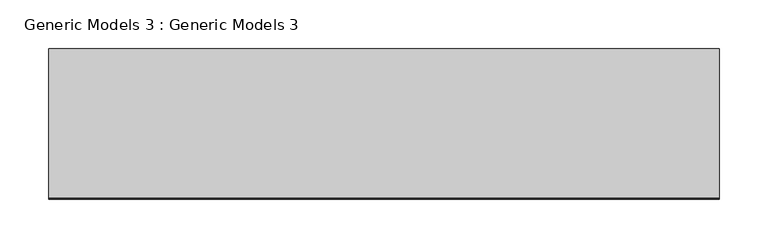
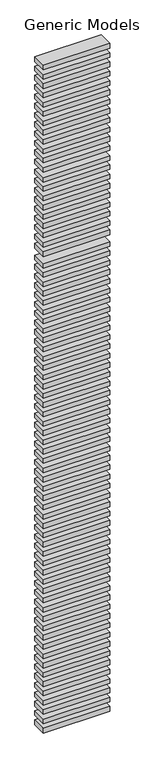
"""IFC4 building model written with IfcOpenShell, lengths in millimetres: proxy geometry, Generic Models 3 : Generic Models 3."""

from ifc_helpers import new_model, si_unit, frame, origin, place, context, project, spatial, polyline, outline, extrude, source, transform, mapped, element, save


def generic_models_3_generic_models_3_1afd715e(model_context):
    return source(origin(), model_context, "Body", "SweptSolid", [
        extrude(outline(polyline([(8219.67371, -13654.3073314), (7533.87371, -13654.3073314), (7533.87371, -13501.9073314), (8219.67371, -13501.9073314), (8219.67371, -13654.3073314)])), frame((0.0, 0.0, 7618.979075), z_axis=(0.0, 0.0, 1.0), x_axis=(1.0, 0.0, 0.0)), (0.0, 0.0, 1.0), 50.8),
        extrude(outline(polyline([(8219.67371, -13654.3073314), (7533.87371, -13654.3073314), (7533.87371, -13501.9073314), (8219.67371, -13501.9073314), (8219.67371, -13654.3073314)])), frame((0.0, 0.0, 7517.379075), z_axis=(0.0, 0.0, 1.0), x_axis=(1.0, 0.0, 0.0)), (0.0, 0.0, 1.0), 50.8),
        extrude(outline(polyline([(8219.67371, -13654.3073314), (7533.87371, -13654.3073314), (7533.87371, -13501.9073314), (8219.67371, -13501.9073314), (8219.67371, -13654.3073314)])), frame((0.0, 0.0, 7415.779075), z_axis=(0.0, 0.0, 1.0), x_axis=(1.0, 0.0, 0.0)), (0.0, 0.0, 1.0), 50.8),
        extrude(outline(polyline([(8219.67371, -13654.3073314), (7533.87371, -13654.3073314), (7533.87371, -13501.9073314), (8219.67371, -13501.9073314), (8219.67371, -13654.3073314)])), frame((0.0, 0.0, 7314.179075), z_axis=(0.0, 0.0, 1.0), x_axis=(1.0, 0.0, 0.0)), (0.0, 0.0, 1.0), 50.8),
        extrude(outline(polyline([(8219.67371, -13654.3073314), (7533.87371, -13654.3073314), (7533.87371, -13501.9073314), (8219.67371, -13501.9073314), (8219.67371, -13654.3073314)])), frame((0.0, 0.0, 7212.579075), z_axis=(0.0, 0.0, 1.0), x_axis=(1.0, 0.0, 0.0)), (0.0, 0.0, 1.0), 50.8),
        extrude(outline(polyline([(8219.67371, -13654.3073314), (7533.87371, -13654.3073314), (7533.87371, -13501.9073314), (8219.67371, -13501.9073314), (8219.67371, -13654.3073314)])), frame((0.0, 0.0, 7110.979075), z_axis=(0.0, 0.0, 1.0), x_axis=(1.0, 0.0, 0.0)), (0.0, 0.0, 1.0), 50.8),
        extrude(outline(polyline([(8219.67371, -13654.3073314), (7533.87371, -13654.3073314), (7533.87371, -13501.9073314), (8219.67371, -13501.9073314), (8219.67371, -13654.3073314)])), frame((0.0, 0.0, 7009.379075), z_axis=(0.0, 0.0, 1.0), x_axis=(1.0, 0.0, 0.0)), (0.0, 0.0, 1.0), 50.8),
        extrude(outline(polyline([(8219.67371, -13654.3073314), (7533.87371, -13654.3073314), (7533.87371, -13501.9073314), (8219.67371, -13501.9073314), (8219.67371, -13654.3073314)])), frame((0.0, 0.0, 6907.779075), z_axis=(0.0, 0.0, 1.0), x_axis=(1.0, 0.0, 0.0)), (0.0, 0.0, 1.0), 50.8),
        extrude(outline(polyline([(8219.67371, -13654.3073314), (7533.87371, -13654.3073314), (7533.87371, -13501.9073314), (8219.67371, -13501.9073314), (8219.67371, -13654.3073314)])), frame((0.0, 0.0, 6806.179075), z_axis=(0.0, 0.0, 1.0), x_axis=(1.0, 0.0, 0.0)), (0.0, 0.0, 1.0), 50.8),
        extrude(outline(polyline([(8219.67371, -13654.3073314), (7533.87371, -13654.3073314), (7533.87371, -13501.9073314), (8219.67371, -13501.9073314), (8219.67371, -13654.3073314)])), frame((0.0, 0.0, 6704.579075), z_axis=(0.0, 0.0, 1.0), x_axis=(1.0, 0.0, 0.0)), (0.0, 0.0, 1.0), 50.8),
        extrude(outline(polyline([(8219.67371, -13654.3073314), (7533.87371, -13654.3073314), (7533.87371, -13501.9073314), (8219.67371, -13501.9073314), (8219.67371, -13654.3073314)])), frame((0.0, 0.0, 6602.979075), z_axis=(0.0, 0.0, 1.0), x_axis=(1.0, 0.0, 0.0)), (0.0, 0.0, 1.0), 50.8),
        extrude(outline(polyline([(8219.67371, -13654.3073314), (7533.87371, -13654.3073314), (7533.87371, -13501.9073314), (8219.67371, -13501.9073314), (8219.67371, -13654.3073314)])), frame((0.0, 0.0, 6501.379075), z_axis=(0.0, 0.0, 1.0), x_axis=(1.0, 0.0, 0.0)), (0.0, 0.0, 1.0), 50.8),
        extrude(outline(polyline([(8219.67371, -13654.3073314), (7533.87371, -13654.3073314), (7533.87371, -13501.9073314), (8219.67371, -13501.9073314), (8219.67371, -13654.3073314)])), frame((0.0, 0.0, 6393.429075), z_axis=(0.0, 0.0, 1.0), x_axis=(1.0, 0.0, 0.0)), (0.0, 0.0, 1.0), 50.8),
        extrude(outline(polyline([(8219.67371, -13654.3073314), (7533.87371, -13654.3073314), (7533.87371, -13501.9073314), (8219.67371, -13501.9073314), (8219.67371, -13654.3073314)])), frame((0.0, 0.0, 6291.829075), z_axis=(0.0, 0.0, 1.0), x_axis=(1.0, 0.0, 0.0)), (0.0, 0.0, 1.0), 50.8),
        extrude(outline(polyline([(8219.67371, -13654.3073314), (7533.87371, -13654.3073314), (7533.87371, -13501.9073314), (8219.67371, -13501.9073314), (8219.67371, -13654.3073314)])), frame((0.0, 0.0, 6190.229075), z_axis=(0.0, 0.0, 1.0), x_axis=(1.0, 0.0, 0.0)), (0.0, 0.0, 1.0), 50.8),
        extrude(outline(polyline([(8219.67371, -13654.3073314), (7533.87371, -13654.3073314), (7533.87371, -13501.9073314), (8219.67371, -13501.9073314), (8219.67371, -13654.3073314)])), frame((0.0, 0.0, 6088.629075), z_axis=(0.0, 0.0, 1.0), x_axis=(1.0, 0.0, 0.0)), (0.0, 0.0, 1.0), 50.8),
        extrude(outline(polyline([(8219.67371, -13654.3073314), (7533.87371, -13654.3073314), (7533.87371, -13501.9073314), (8219.67371, -13501.9073314), (8219.67371, -13654.3073314)])), frame((0.0, 0.0, 5987.029075), z_axis=(0.0, 0.0, 1.0), x_axis=(1.0, 0.0, 0.0)), (0.0, 0.0, 1.0), 50.8),
        extrude(outline(polyline([(8219.67371, -13654.3073314), (7533.87371, -13654.3073314), (7533.87371, -13501.9073314), (8219.67371, -13501.9073314), (8219.67371, -13654.3073314)])), frame((0.0, 0.0, 5885.429075), z_axis=(0.0, 0.0, 1.0), x_axis=(1.0, 0.0, 0.0)), (0.0, 0.0, 1.0), 50.8),
        extrude(outline(polyline([(8219.67371, -13654.3073314), (7533.87371, -13654.3073314), (7533.87371, -13501.9073314), (8219.67371, -13501.9073314), (8219.67371, -13654.3073314)])), frame((0.0, 0.0, 5783.829075), z_axis=(0.0, 0.0, 1.0), x_axis=(1.0, 0.0, 0.0)), (0.0, 0.0, 1.0), 50.8),
        extrude(outline(polyline([(8219.67371, -13654.3073314), (7533.87371, -13654.3073314), (7533.87371, -13501.9073314), (8219.67371, -13501.9073314), (8219.67371, -13654.3073314)])), frame((0.0, 0.0, 5682.229075), z_axis=(0.0, 0.0, 1.0), x_axis=(1.0, 0.0, 0.0)), (0.0, 0.0, 1.0), 50.8),
        extrude(outline(polyline([(8219.67371, -13654.3073314), (7533.87371, -13654.3073314), (7533.87371, -13501.9073314), (8219.67371, -13501.9073314), (8219.67371, -13654.3073314)])), frame((0.0, 0.0, 5580.629075), z_axis=(0.0, 0.0, 1.0), x_axis=(1.0, 0.0, 0.0)), (0.0, 0.0, 1.0), 50.8),
        extrude(outline(polyline([(8219.67371, -13654.3073314), (7533.87371, -13654.3073314), (7533.87371, -13501.9073314), (8219.67371, -13501.9073314), (8219.67371, -13654.3073314)])), frame((0.0, 0.0, 5453.629075), z_axis=(0.0, 0.0, 1.0), x_axis=(1.0, 0.0, 0.0)), (0.0, 0.0, 1.0), 50.8),
        extrude(outline(polyline([(8219.67371, -13654.3073314), (7533.87371, -13654.3073314), (7533.87371, -13501.9073314), (8219.67371, -13501.9073314), (8219.67371, -13654.3073314)])), frame((0.0, 0.0, 5352.029075), z_axis=(0.0, 0.0, 1.0), x_axis=(1.0, 0.0, 0.0)), (0.0, 0.0, 1.0), 50.8),
        extrude(outline(polyline([(8219.67371, -13654.3073314), (7533.87371, -13654.3073314), (7533.87371, -13501.9073314), (8219.67371, -13501.9073314), (8219.67371, -13654.3073314)])), frame((0.0, 0.0, 5250.429075), z_axis=(0.0, 0.0, 1.0), x_axis=(1.0, 0.0, 0.0)), (0.0, 0.0, 1.0), 50.8),
        extrude(outline(polyline([(8219.67371, -13654.3073314), (7533.87371, -13654.3073314), (7533.87371, -13501.9073314), (8219.67371, -13501.9073314), (8219.67371, -13654.3073314)])), frame((0.0, 0.0, 5148.829075), z_axis=(0.0, 0.0, 1.0), x_axis=(1.0, 0.0, 0.0)), (0.0, 0.0, 1.0), 50.8),
        extrude(outline(polyline([(8219.67371, -13654.3073314), (7533.87371, -13654.3073314), (7533.87371, -13501.9073314), (8219.67371, -13501.9073314), (8219.67371, -13654.3073314)])), frame((0.0, 0.0, 5047.229075), z_axis=(0.0, 0.0, 1.0), x_axis=(1.0, 0.0, 0.0)), (0.0, 0.0, 1.0), 50.8),
        extrude(outline(polyline([(8219.67371, -13654.3073314), (7533.87371, -13654.3073314), (7533.87371, -13501.9073314), (8219.67371, -13501.9073314), (8219.67371, -13654.3073314)])), frame((0.0, 0.0, 4945.629075), z_axis=(0.0, 0.0, 1.0), x_axis=(1.0, 0.0, 0.0)), (0.0, 0.0, 1.0), 50.8),
        extrude(outline(polyline([(8219.67371, -13654.3073314), (7533.87371, -13654.3073314), (7533.87371, -13501.9073314), (8219.67371, -13501.9073314), (8219.67371, -13654.3073314)])), frame((0.0, 0.0, 4844.029075), z_axis=(0.0, 0.0, 1.0), x_axis=(1.0, 0.0, 0.0)), (0.0, 0.0, 1.0), 50.8),
        extrude(outline(polyline([(8219.67371, -13654.3073314), (7533.87371, -13654.3073314), (7533.87371, -13501.9073314), (8219.67371, -13501.9073314), (8219.67371, -13654.3073314)])), frame((0.0, 0.0, 4742.429075), z_axis=(0.0, 0.0, 1.0), x_axis=(1.0, 0.0, 0.0)), (0.0, 0.0, 1.0), 50.8),
        extrude(outline(polyline([(8219.67371, -13654.3073314), (7533.87371, -13654.3073314), (7533.87371, -13501.9073314), (8219.67371, -13501.9073314), (8219.67371, -13654.3073314)])), frame((0.0, 0.0, 4640.829075), z_axis=(0.0, 0.0, 1.0), x_axis=(1.0, 0.0, 0.0)), (0.0, 0.0, 1.0), 50.8),
        extrude(outline(polyline([(8219.67371, -13654.3073314), (7533.87371, -13654.3073314), (7533.87371, -13501.9073314), (8219.67371, -13501.9073314), (8219.67371, -13654.3073314)])), frame((0.0, 0.0, 4539.229075), z_axis=(0.0, 0.0, 1.0), x_axis=(1.0, 0.0, 0.0)), (0.0, 0.0, 1.0), 50.8),
        extrude(outline(polyline([(8219.67371, -13654.3073314), (7533.87371, -13654.3073314), (7533.87371, -13501.9073314), (8219.67371, -13501.9073314), (8219.67371, -13654.3073314)])), frame((0.0, 0.0, 4437.629075), z_axis=(0.0, 0.0, 1.0), x_axis=(1.0, 0.0, 0.0)), (0.0, 0.0, 1.0), 50.8),
        extrude(outline(polyline([(8219.67371, -13654.3073314), (7533.87371, -13654.3073314), (7533.87371, -13501.9073314), (8219.67371, -13501.9073314), (8219.67371, -13654.3073314)])), frame((0.0, 0.0, 4336.029075), z_axis=(0.0, 0.0, 1.0), x_axis=(1.0, 0.0, 0.0)), (0.0, 0.0, 1.0), 50.8),
        extrude(outline(polyline([(8219.67371, -13654.3073314), (7533.87371, -13654.3073314), (7533.87371, -13501.9073314), (8219.67371, -13501.9073314), (8219.67371, -13654.3073314)])), frame((0.0, 0.0, 4234.429075), z_axis=(0.0, 0.0, 1.0), x_axis=(1.0, 0.0, 0.0)), (0.0, 0.0, 1.0), 50.8),
        extrude(outline(polyline([(8219.67371, -13654.3073314), (7533.87371, -13654.3073314), (7533.87371, -13501.9073314), (8219.67371, -13501.9073314), (8219.67371, -13654.3073314)])), frame((0.0, 0.0, 4132.829075), z_axis=(0.0, 0.0, 1.0), x_axis=(1.0, 0.0, 0.0)), (0.0, 0.0, 1.0), 50.8),
        extrude(outline(polyline([(8219.67371, -13654.3073314), (7533.87371, -13654.3073314), (7533.87371, -13501.9073314), (8219.67371, -13501.9073314), (8219.67371, -13654.3073314)])), frame((0.0, 0.0, 4031.229075), z_axis=(0.0, 0.0, 1.0), x_axis=(1.0, 0.0, 0.0)), (0.0, 0.0, 1.0), 50.8),
        extrude(outline(polyline([(8219.67371, -13654.3073314), (7533.87371, -13654.3073314), (7533.87371, -13501.9073314), (8219.67371, -13501.9073314), (8219.67371, -13654.3073314)])), frame((0.0, 0.0, 3929.629075), z_axis=(0.0, 0.0, 1.0), x_axis=(1.0, 0.0, 0.0)), (0.0, 0.0, 1.0), 50.8),
        extrude(outline(polyline([(8219.67371, -13654.3073314), (7533.87371, -13654.3073314), (7533.87371, -13501.9073314), (8219.67371, -13501.9073314), (8219.67371, -13654.3073314)])), frame((0.0, 0.0, 3828.029075), z_axis=(0.0, 0.0, 1.0), x_axis=(1.0, 0.0, 0.0)), (0.0, 0.0, 1.0), 50.8),
        extrude(outline(polyline([(8219.67371, -13654.3073314), (7533.87371, -13654.3073314), (7533.87371, -13501.9073314), (8219.67371, -13501.9073314), (8219.67371, -13654.3073314)])), frame((0.0, 0.0, 3726.429075), z_axis=(0.0, 0.0, 1.0), x_axis=(1.0, 0.0, 0.0)), (0.0, 0.0, 1.0), 50.8),
        extrude(outline(polyline([(8219.67371, -13654.3073314), (7533.87371, -13654.3073314), (7533.87371, -13501.9073314), (8219.67371, -13501.9073314), (8219.67371, -13654.3073314)])), frame((0.0, 0.0, 3624.829075), z_axis=(0.0, 0.0, 1.0), x_axis=(1.0, 0.0, 0.0)), (0.0, 0.0, 1.0), 50.8),
        extrude(outline(polyline([(8219.67371, -13654.3073314), (7533.87371, -13654.3073314), (7533.87371, -13501.9073314), (8219.67371, -13501.9073314), (8219.67371, -13654.3073314)])), frame((0.0, 0.0, 3523.229075), z_axis=(0.0, 0.0, 1.0), x_axis=(1.0, 0.0, 0.0)), (0.0, 0.0, 1.0), 50.8),
        extrude(outline(polyline([(8219.67371, -13654.3073314), (7533.87371, -13654.3073314), (7533.87371, -13501.9073314), (8219.67371, -13501.9073314), (8219.67371, -13654.3073314)])), frame((0.0, 0.0, 3421.629075), z_axis=(0.0, 0.0, 1.0), x_axis=(1.0, 0.0, 0.0)), (0.0, 0.0, 1.0), 50.8),
        extrude(outline(polyline([(8219.67371, -13654.3073314), (7533.87371, -13654.3073314), (7533.87371, -13501.9073314), (8219.67371, -13501.9073314), (8219.67371, -13654.3073314)])), frame((0.0, 0.0, 3320.029075), z_axis=(0.0, 0.0, 1.0), x_axis=(1.0, 0.0, 0.0)), (0.0, 0.0, 1.0), 50.8),
        extrude(outline(polyline([(8219.67371, -13654.3073314), (7533.87371, -13654.3073314), (7533.87371, -13501.9073314), (8219.67371, -13501.9073314), (8219.67371, -13654.3073314)])), frame((0.0, 0.0, 3218.429075), z_axis=(0.0, 0.0, 1.0), x_axis=(1.0, 0.0, 0.0)), (0.0, 0.0, 1.0), 50.8),
        extrude(outline(polyline([(8219.67371, -13654.3073314), (7533.87371, -13654.3073314), (7533.87371, -13501.9073314), (8219.67371, -13501.9073314), (8219.67371, -13654.3073314)])), frame((0.0, 0.0, 3116.829075), z_axis=(0.0, 0.0, 1.0), x_axis=(1.0, 0.0, 0.0)), (0.0, 0.0, 1.0), 50.8),
        extrude(outline(polyline([(8219.67371, -13654.3073314), (7533.87371, -13654.3073314), (7533.87371, -13501.9073314), (8219.67371, -13501.9073314), (8219.67371, -13654.3073314)])), frame((0.0, 0.0, 3015.229075), z_axis=(0.0, 0.0, 1.0), x_axis=(1.0, 0.0, 0.0)), (0.0, 0.0, 1.0), 50.8),
        extrude(outline(polyline([(8219.67371, -13654.3073314), (7533.87371, -13654.3073314), (7533.87371, -13501.9073314), (8219.67371, -13501.9073314), (8219.67371, -13654.3073314)])), frame((0.0, 0.0, 2913.629075), z_axis=(0.0, 0.0, 1.0), x_axis=(1.0, 0.0, 0.0)), (0.0, 0.0, 1.0), 50.8),
        extrude(outline(polyline([(8219.67371, -13654.3073314), (7533.87371, -13654.3073314), (7533.87371, -13501.9073314), (8219.67371, -13501.9073314), (8219.67371, -13654.3073314)])), frame((0.0, 0.0, 2812.029075), z_axis=(0.0, 0.0, 1.0), x_axis=(1.0, 0.0, 0.0)), (0.0, 0.0, 1.0), 50.8),
        extrude(outline(polyline([(8219.67371, -13654.3073314), (7533.87371, -13654.3073314), (7533.87371, -13501.9073314), (8219.67371, -13501.9073314), (8219.67371, -13654.3073314)])), frame((0.0, 0.0, 2710.429075), z_axis=(0.0, 0.0, 1.0), x_axis=(1.0, 0.0, 0.0)), (0.0, 0.0, 1.0), 50.8),
        extrude(outline(polyline([(8219.67371, -13654.3073314), (7533.87371, -13654.3073314), (7533.87371, -13501.9073314), (8219.67371, -13501.9073314), (8219.67371, -13654.3073314)])), frame((0.0, 0.0, 2608.829075), z_axis=(0.0, 0.0, 1.0), x_axis=(1.0, 0.0, 0.0)), (0.0, 0.0, 1.0), 50.8),
        extrude(outline(polyline([(8219.67371, -13654.3073314), (7533.87371, -13654.3073314), (7533.87371, -13501.9073314), (8219.67371, -13501.9073314), (8219.67371, -13654.3073314)])), frame((0.0, 0.0, 2507.229075), z_axis=(0.0, 0.0, 1.0), x_axis=(1.0, 0.0, 0.0)), (0.0, 0.0, 1.0), 50.8),
        extrude(outline(polyline([(8219.67371, -13654.3073314), (7533.87371, -13654.3073314), (7533.87371, -13501.9073314), (8219.67371, -13501.9073314), (8219.67371, -13654.3073314)])), frame((0.0, 0.0, 2405.629075), z_axis=(0.0, 0.0, 1.0), x_axis=(1.0, 0.0, 0.0)), (0.0, 0.0, 1.0), 50.8),
        extrude(outline(polyline([(8219.67371, -13654.3073314), (7533.87371, -13654.3073314), (7533.87371, -13501.9073314), (8219.67371, -13501.9073314), (8219.67371, -13654.3073314)])), frame((0.0, 0.0, 2304.029075), z_axis=(0.0, 0.0, 1.0), x_axis=(1.0, 0.0, 0.0)), (0.0, 0.0, 1.0), 50.8),
        extrude(outline(polyline([(8219.67371, -13654.3073314), (7533.87371, -13654.3073314), (7533.87371, -13501.9073314), (8219.67371, -13501.9073314), (8219.67371, -13654.3073314)])), frame((0.0, 0.0, 2202.429075), z_axis=(0.0, 0.0, 1.0), x_axis=(1.0, 0.0, 0.0)), (0.0, 0.0, 1.0), 50.8),
        extrude(outline(polyline([(8219.67371, -13654.3073314), (7533.87371, -13654.3073314), (7533.87371, -13501.9073314), (8219.67371, -13501.9073314), (8219.67371, -13654.3073314)])), frame((0.0, 0.0, 2100.829075), z_axis=(0.0, 0.0, 1.0), x_axis=(1.0, 0.0, 0.0)), (0.0, 0.0, 1.0), 50.8),
        extrude(outline(polyline([(8219.67371, -13654.3073314), (7533.87371, -13654.3073314), (7533.87371, -13501.9073314), (8219.67371, -13501.9073314), (8219.67371, -13654.3073314)])), frame((0.0, 0.0, 1999.229075), z_axis=(0.0, 0.0, 1.0), x_axis=(1.0, 0.0, 0.0)), (0.0, 0.0, 1.0), 50.8),
        extrude(outline(polyline([(8219.67371, -13654.3073314), (7533.87371, -13654.3073314), (7533.87371, -13501.9073314), (8219.67371, -13501.9073314), (8219.67371, -13654.3073314)])), frame((0.0, 0.0, 1897.629075), z_axis=(0.0, 0.0, 1.0), x_axis=(1.0, 0.0, 0.0)), (0.0, 0.0, 1.0), 50.8),
        extrude(outline(polyline([(8219.67371, -13654.3073314), (7533.87371, -13654.3073314), (7533.87371, -13501.9073314), (8219.67371, -13501.9073314), (8219.67371, -13654.3073314)])), frame((0.0, 0.0, 1796.029075), z_axis=(0.0, 0.0, 1.0), x_axis=(1.0, 0.0, 0.0)), (0.0, 0.0, 1.0), 50.8),
        extrude(outline(polyline([(8219.67371, -13654.3073314), (7533.87371, -13654.3073314), (7533.87371, -13501.9073314), (8219.67371, -13501.9073314), (8219.67371, -13654.3073314)])), frame((0.0, 0.0, 1694.429075), z_axis=(0.0, 0.0, 1.0), x_axis=(1.0, 0.0, 0.0)), (0.0, 0.0, 1.0), 50.8),
        extrude(outline(polyline([(8219.67371, -13654.3073314), (7533.87371, -13654.3073314), (7533.87371, -13501.9073314), (8219.67371, -13501.9073314), (8219.67371, -13654.3073314)])), frame((0.0, 0.0, 1592.829075), z_axis=(0.0, 0.0, 1.0), x_axis=(1.0, 0.0, 0.0)), (0.0, 0.0, 1.0), 50.8),
        extrude(outline(polyline([(8219.67371, -13654.3073314), (7533.87371, -13654.3073314), (7533.87371, -13501.9073314), (8219.67371, -13501.9073314), (8219.67371, -13654.3073314)])), frame((0.0, 0.0, 1491.229075), z_axis=(0.0, 0.0, 1.0), x_axis=(1.0, 0.0, 0.0)), (0.0, 0.0, 1.0), 50.8),
        extrude(outline(polyline([(8219.67371, -13654.3073314), (7533.87371, -13654.3073314), (7533.87371, -13501.9073314), (8219.67371, -13501.9073314), (8219.67371, -13654.3073314)])), frame((0.0, 0.0, 1389.629075), z_axis=(0.0, 0.0, 1.0), x_axis=(1.0, 0.0, 0.0)), (0.0, 0.0, 1.0), 50.8),
        extrude(outline(polyline([(8219.67371, -13654.3073314), (7533.87371, -13654.3073314), (7533.87371, -13501.9073314), (8219.67371, -13501.9073314), (8219.67371, -13654.3073314)])), frame((0.0, 0.0, 1288.029075), z_axis=(0.0, 0.0, 1.0), x_axis=(1.0, 0.0, 0.0)), (0.0, 0.0, 1.0), 50.8),
        extrude(outline(polyline([(8219.67371, -13654.3073314), (7533.87371, -13654.3073314), (7533.87371, -13501.9073314), (8219.67371, -13501.9073314), (8219.67371, -13654.3073314)])), frame((0.0, 0.0, 1186.429075), z_axis=(0.0, 0.0, 1.0), x_axis=(1.0, 0.0, 0.0)), (0.0, 0.0, 1.0), 50.8),
        extrude(outline(polyline([(8219.67371, -13654.3073314), (7533.87371, -13654.3073314), (7533.87371, -13501.9073314), (8219.67371, -13501.9073314), (8219.67371, -13654.3073314)])), frame((0.0, 0.0, 1084.829075), z_axis=(0.0, 0.0, 1.0), x_axis=(1.0, 0.0, 0.0)), (0.0, 0.0, 1.0), 50.8),
        extrude(outline(polyline([(8219.67371, -13654.3073314), (7533.87371, -13654.3073314), (7533.87371, -13501.9073314), (8219.67371, -13501.9073314), (8219.67371, -13654.3073314)])), frame((0.0, 0.0, 983.229075), z_axis=(0.0, 0.0, 1.0), x_axis=(1.0, 0.0, 0.0)), (0.0, 0.0, 1.0), 50.8),
        extrude(outline(polyline([(8219.67371, -13654.3073314), (7533.87371, -13654.3073314), (7533.87371, -13501.9073314), (8219.67371, -13501.9073314), (8219.67371, -13654.3073314)])), frame((0.0, 0.0, 881.629075), z_axis=(0.0, 0.0, 1.0), x_axis=(1.0, 0.0, 0.0)), (0.0, 0.0, 1.0), 50.8),
        extrude(outline(polyline([(8219.67371, -13654.3073314), (7533.87371, -13654.3073314), (7533.87371, -13501.9073314), (8219.67371, -13501.9073314), (8219.67371, -13654.3073314)])), frame((0.0, 0.0, 780.029075), z_axis=(0.0, 0.0, 1.0), x_axis=(1.0, 0.0, 0.0)), (0.0, 0.0, 1.0), 50.8),
        extrude(outline(polyline([(8219.67371, -13654.3073314), (7533.87371, -13654.3073314), (7533.87371, -13501.9073314), (8219.67371, -13501.9073314), (8219.67371, -13654.3073314)])), frame((0.0, 0.0, 678.429075), z_axis=(0.0, 0.0, 1.0), x_axis=(1.0, 0.0, 0.0)), (0.0, 0.0, 1.0), 50.8),
        extrude(outline(polyline([(8219.67371, -13654.3073314), (7533.87371, -13654.3073314), (7533.87371, -13501.9073314), (8219.67371, -13501.9073314), (8219.67371, -13654.3073314)])), frame((0.0, 0.0, 576.829075), z_axis=(0.0, 0.0, 1.0), x_axis=(1.0, 0.0, 0.0)), (0.0, 0.0, 1.0), 50.8),
        extrude(outline(polyline([(8219.67371, -13654.3073314), (7533.87371, -13654.3073314), (7533.87371, -13501.9073314), (8219.67371, -13501.9073314), (8219.67371, -13654.3073314)])), frame((0.0, 0.0, 475.229075), z_axis=(0.0, 0.0, 1.0), x_axis=(1.0, 0.0, 0.0)), (0.0, 0.0, 1.0), 50.8),
        extrude(outline(polyline([(8219.67371, -13654.3073314), (7533.87371, -13654.3073314), (7533.87371, -13501.9073314), (8219.67371, -13501.9073314), (8219.67371, -13654.3073314)])), frame((0.0, 0.0, 373.629075), z_axis=(0.0, 0.0, 1.0), x_axis=(1.0, 0.0, 0.0)), (0.0, 0.0, 1.0), 50.8),
    ])


if __name__ == "__main__":
    model = new_model("IFC4")
    model_context = context("Model", 3, world=origin())
    ifc_project = project(units=[si_unit("LENGTHUNIT", "METRE", prefix="MILLI")], contexts=[model_context])
    site = spatial("IfcSite", under=ifc_project)
    building = spatial("IfcBuilding", under=site)
    placement = place(None, origin())
    generic_models_3_generic_models_3_shape = generic_models_3_generic_models_3_1afd715e(model_context)
    element("IfcBuildingElementProxy", 1, Name="Generic Models 3 : Generic Models 3", ObjectType="Generic Models 3 : Generic Models 3", at=placement, inside=building, context=model_context, shape_type="MappedRepresentation", body=[
        mapped(generic_models_3_generic_models_3_shape, transform((0.0, 0.0, 0.0), x_axis=(1.0, 0.0, 0.0), y_axis=(0.0, 1.0, 0.0), z_axis=(0.0, 0.0, 1.0))),
    ])
    save(model, "model.ifc")

# Revit data of these elements
# Element 1 (IfcBuildingElementProxy, "Generic Models 3 : Generic Models 3")
#   Materials on its faces: "WOOD MATERIAL 9\""
# Materials
#   "WOOD MATERIAL 9\"": class "Generic", colour RGB 120 120 120, transparency 0, Cost = 0
